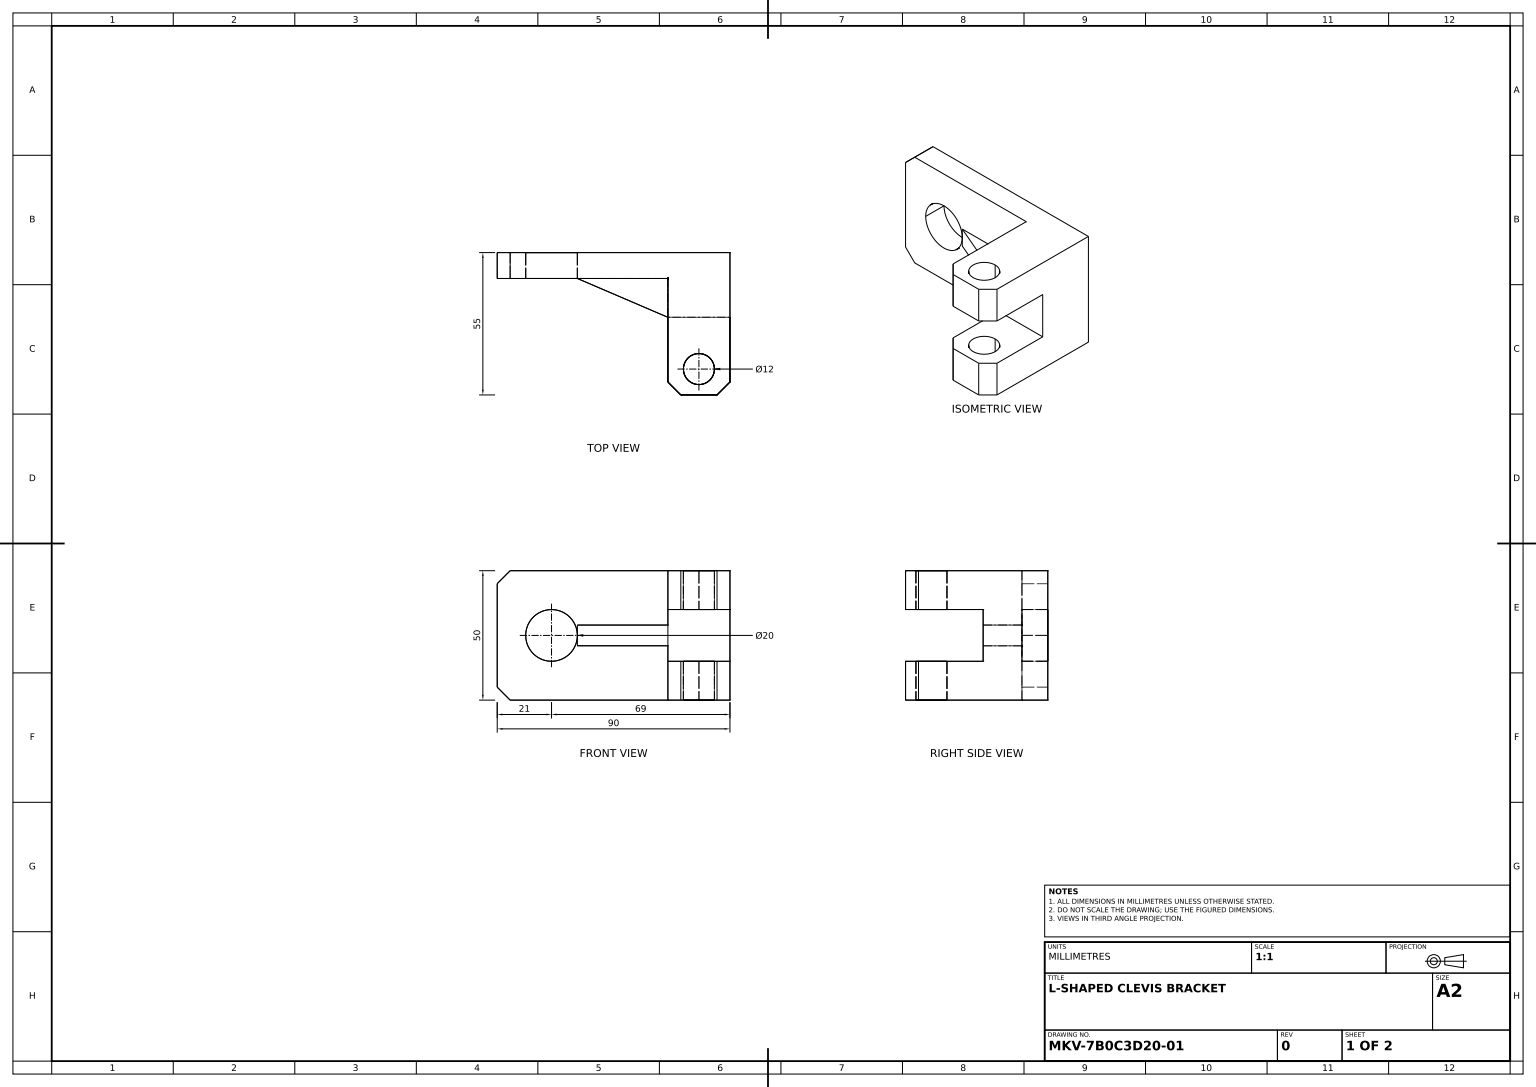
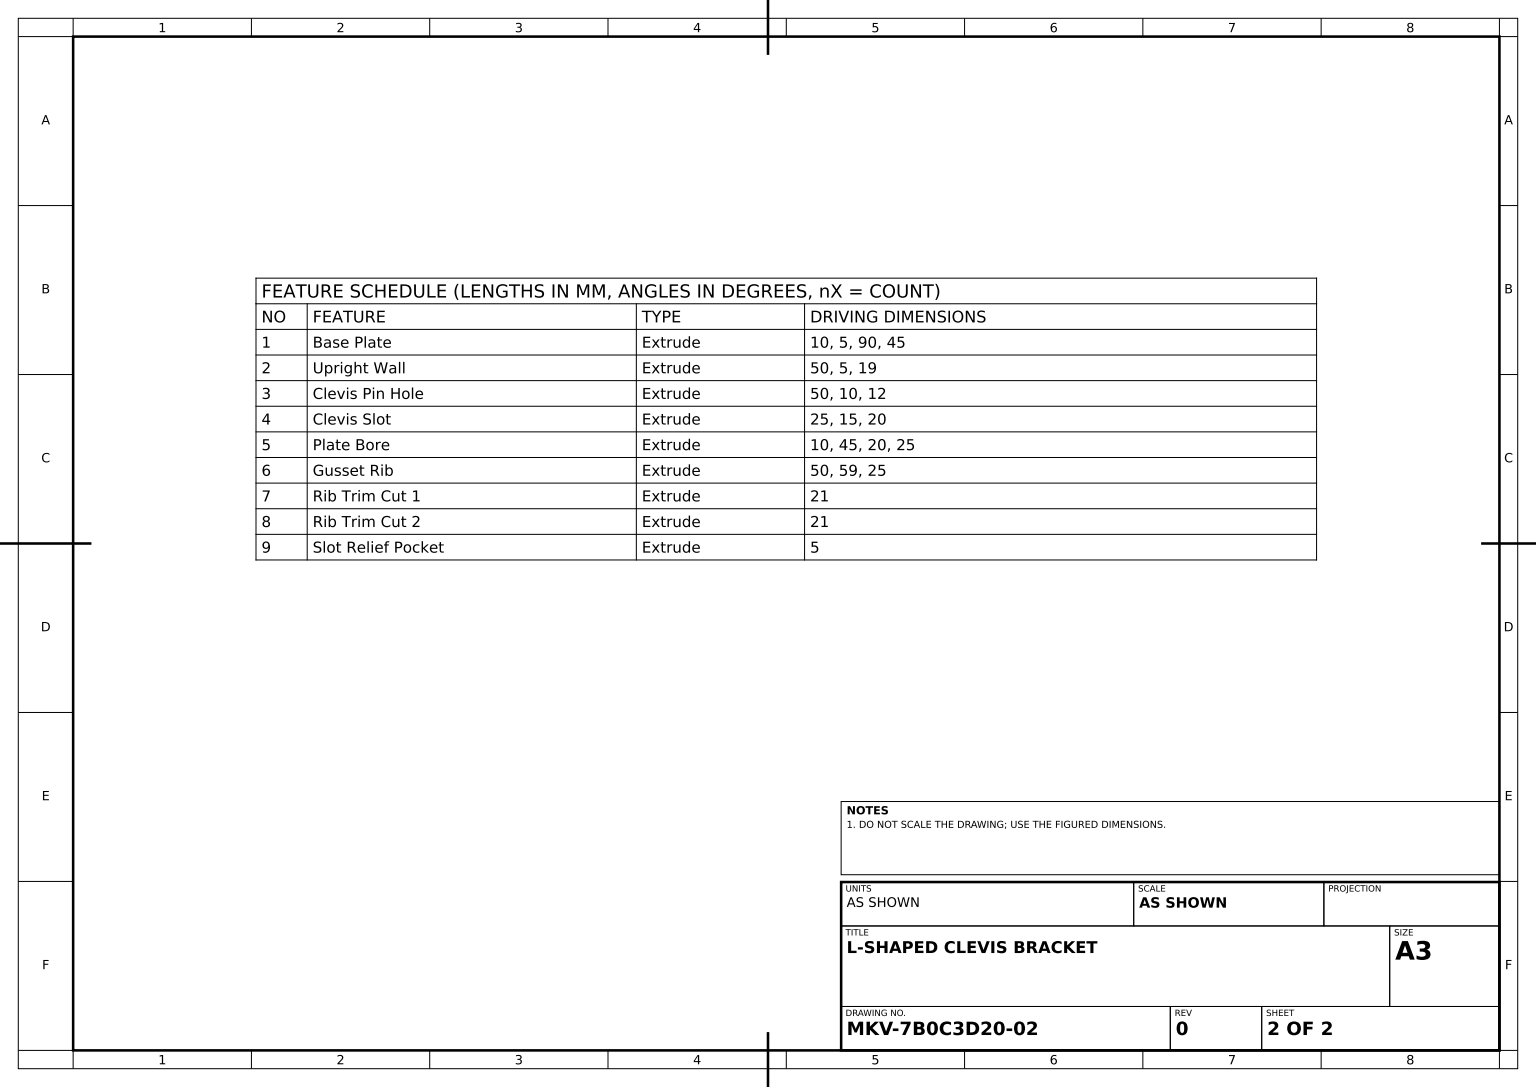
SolidWorks part; units mm, degrees
material "Plain Carbon Steel"
ref_plane "Front Plane" through (0, 0, 0) normal (0, 0, 1) x (1, 0, 0)
ref_plane "Top Plane" through (0, 0, 0) normal (0, 1, 0) x (1, 0, 0)
ref_plane "Right Plane" through (0, 0, 0) normal (1, 0, 0) x (0, 0, -1)
sketch "Base Plate Profile" plane through (0, 0, 0) normal (0, 0, 1) x (1, 0, 0)
  line L0 (90, 0) -> (5, 0)
  line L1 (90, 0) -> (90, 50)
  line L2 (90, 50) -> (5, 50)
  line L5 (0, 45) -> (0, 5)
  line L6 (0, 5) -> (5, 0)
  line L7 (0, 45) -> (5, 50)
  dimension "D1" = 5
  dimension "D2" = 90
  dimension "D3" = 5
  dimension "D4" = 45
extrude "Base Plate" add sketch "Base Plate Profile" along normal blind 10
sketch "Upright Wall Profile" plane through (0, 0, 0) normal (0, -1, 0) x (1, 0, 0)
  line L0 (90, 10) -> (90, 50)
  line L6 (90, 10) -> (90, 0) construction
  line L10 (66, 50) -> (66, 10)
  line L11 (5, 10) -> (90, 10) construction
  line L12 (66, 10) -> (90, 10)
  line L14 (71, 55) -> (66, 50)
  line L15 (85, 55) -> (90, 50)
  line L16 (71, 55) -> (85, 55)
  line L17 (5, 0) -> (90, 0) construction
  dimension "D1" = 5
  dimension "D2" = 19
  dimension "D3" = 50
extrude "Upright Wall" add sketch "Upright Wall Profile" against normal blind 50
sketch "Clevis Pin Hole Sketch" plane through (0, 0, 0) normal (0, -1, 0) x (1, 0, 0)
  line L0 (85, 55) -> (71, 55) construction
  line L1 (90, 50) -> (90, 0) construction
  circle A1 centre (78, 45) radius 6
  dimension "D1" = 10
  dimension "D2" = 12
  dimension "D3" = 12
  dimension "D4" = 12
extrude "Clevis Pin Hole" cut sketch "Clevis Pin Hole Sketch" against normal blind 50
sketch "Clevis Slot Sketch" plane through (0, 0, 55) normal (0, 0, 1) x (1, 0, 0)
  line L0 (66, 50) -> (66, 0) construction
  line L1 (66, 35) -> (90, 35)
  line L2 (66, 35) -> (66, 15)
  line L3 (66, 15) -> (90, 15)
  line L4 (90, 35) -> (90, 15)
  line L5 (90, 50) -> (90, 0) construction
  line L6 (85, 50) -> (71, 50) construction
  dimension "D1" = 15
  dimension "D2" = 20
extrude "Clevis Slot" cut sketch "Clevis Slot Sketch" against normal blind 25
sketch "Plate Bore Sketch" plane through (0, 0, 10) normal (0, 0, 1) x (1, 0, 0)
  line L0 (66, 50) -> (66, 35) construction
  line L2 (66, 50) -> (5, 50) construction
  circle A0 centre (21, 25) radius 10
  dimension "D1" = 20
  dimension "D3" = 20
  dimension "D2" = 45
  dimension "D4" = 25
extrude "Plate Bore" cut sketch "Plate Bore Sketch" against normal blind 10
sketch "Gusset Rib Profile" plane through (0, 0, 0) normal (0, -1, 0) x (1, 0, 0)
  line L0 (66, 10) -> (66, 25)
  line L1 (66, 50) -> (66, 10) construction
  line L2 (66, 10) -> (31, 10)
  line L3 (5, 10) -> (66, 10) construction
  line L4 (31, 10) -> (66, 25)
  line L5 (90, 50) -> (90, 0) construction
  line L6 (5, 0) -> (90, 0) construction
  dimension "D1" = 59
  dimension "D2" = 25
extrude "Gusset Rib" add sketch "Gusset Rib Profile" against normal blind 50
sketch "Rib Trim Cut 1 Sketch" plane through (0, 0, 0) normal (0, -1, 0) x (1, 0, 0)
  line L0 (66, 25) -> (66, 10)
  line L1 (66, 10) -> (31, 10)
  line L2 (31, 10) -> (66, 25)
extrude "Rib Trim Cut 1" cut sketch "Rib Trim Cut 1 Sketch" against normal blind 21
sketch "Rib Trim Cut 2 Sketch" plane through (0, 50, 0) normal (0, 1, 0) x (1, 0, 0)
  line L0 (66, -25) -> (66, -10)
  line L1 (66, -10) -> (31, -10)
  line L2 (31, -10) -> (66, -25)
extrude "Rib Trim Cut 2" cut sketch "Rib Trim Cut 2 Sketch" against normal blind 21
sketch "Slot Relief Pocket Sketch" plane through (0, 0, 30) normal (0, 0, 1) x (1, 0, 0)
  line L0 (90, 35) -> (90, 15)
  line L1 (90, 15) -> (66, 15)
  line L2 (66, 15) -> (66, 35)
  line L3 (66, 35) -> (90, 35)
extrude "Slot Relief Pocket" cut sketch "Slot Relief Pocket Sketch" against normal blind 5
